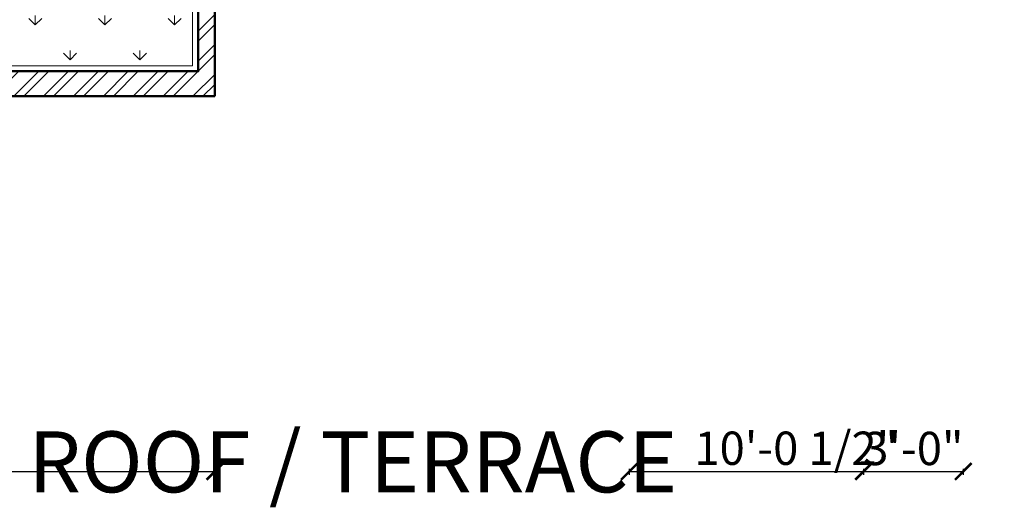
# Model space of a CAD drawing. Units: inches. Extents: x 261 to 2725, y 291 to 1454.
# Tile 27 of 35: x 2144 to 2500, y 291 to 467. Entities that reach past the tile are written whole.
import ezdxf

# ---------------------------------------------------------------- set-up
doc = ezdxf.new("R2010")
doc.units = ezdxf.units.IN
for name, color, linetype, lineweight in [('A-ANNO-DIMS', 136, 'Continuous', 18), ('A-ANNO-TEXT', 7, 'Continuous', 25), ('A-PLNT', 3, 'Continuous', 18), ('A-PLNT-PATT', 3, 'Continuous', 13), ('A-WALL', 222, 'Continuous', 50), ('A-WALL-PATT', 243, 'Continuous', 13)]:
    doc.layers.add(name, color=color, linetype=linetype, lineweight=lineweight)
doc.styles.get("Standard").update_dxf_attribs({"font": 'arial.ttf'})
doc.dimstyles.new('ISO-25', dxfattribs={"dimtxt": 12, "dimasz": 6, "dimexe": 1.25, "dimexo": 0.625, "dimtad": 1, "dimdec": 0, "dimlunit": 3, "dimtxsty": 'Standard', "dimblk": 'ARCHTICK', "dimcen": 2.5, "dimadec": 0, "dimazin": 0, "dimtfac": 1, "dimtdec": 0, "dimtmove": 0, "dimatfit": 3, "dimfxl": 1, "dimfxlon": 1, "dimarcsym": 0})

# ---------------------------------------------------------------- blocks, each defined once
blk = doc.blocks.new('_ArchTick')
at = {"color": 0, "linetype": 'ByBlock', "const_width": 0.15}
blk.add_lwpolyline([(-0.5, -0.5), (0.5, 0.5)], dxfattribs=at)
blk = doc.blocks.new('*D89')
at = {"layer": 'A-ANNO-DIMS', "color": 0, "lineweight": -2, "ltscale": 0.07, "transparency": 16777216}
for p, q in [((2600.96, 508.47), (2603.21, 508.47)), ((2601.96, 412.47), (2601.96, 508.47)), ((2600.96, 412.47), (2603.21, 412.47))]:
    blk.add_line(p, q, dxfattribs=at)
at = {"layer": 'Defpoints', "color": 0, "ltscale": 0.07, "transparency": 16777216}
for p in [(955.45, 508.47), (2601.96, 508.47), (994.45, 412.47)]:
    blk.add_point(p, dxfattribs=at)
at = {"layer": 'A-ANNO-DIMS', "color": 0, "lineweight": -2, "ltscale": 0.07, "transparency": 16777216, "xscale": 6, "yscale": 6, "zscale": 6}
for p, rotation in [((2601.96, 508.47), 90), ((2601.96, 412.47), 270)]:
    blk.add_blockref('_ArchTick', p, dxfattribs=dict(at, rotation=rotation))
at = {"layer": 'A-ANNO-DIMS', "color": 0, "ltscale": 0.07, "transparency": 16777216, "insert": (2595.21, 460.47), "char_height": 12, "attachment_point": 5, "rotation": 90}
blk.add_mtext('8\'-0"', dxfattribs=at)
blk = doc.blocks.new('*D111')
at = {"layer": 'A-ANNO-DIMS', "color": 0, "lineweight": -2, "ltscale": 0.07, "transparency": 16777216}
for p, q in [((2600.96, 550.47), (2603.21, 550.47)), ((2601.96, 448.47), (2601.96, 550.47)), ((2600.96, 448.47), (2603.21, 448.47))]:
    blk.add_line(p, q, dxfattribs=at)
at = {"layer": 'Defpoints', "color": 0, "ltscale": 0.07, "transparency": 16777216}
for p in [(1720.08, 550.47), (2601.96, 550.47), (1720.08, 448.47)]:
    blk.add_point(p, dxfattribs=at)
at = {"layer": 'A-ANNO-DIMS', "color": 0, "lineweight": -2, "ltscale": 0.07, "transparency": 16777216, "xscale": 6, "yscale": 6, "zscale": 6}
for p, rotation in [((2601.96, 550.47), 90), ((2601.96, 448.47), 270)]:
    blk.add_blockref('_ArchTick', p, dxfattribs=dict(at, rotation=rotation))
at = {"layer": 'A-ANNO-DIMS', "color": 0, "ltscale": 0.07, "transparency": 16777216, "insert": (2595.21, 499.47), "char_height": 12, "attachment_point": 5, "rotation": 90}
blk.add_mtext('8\'-6"', dxfattribs=at)
blk = doc.blocks.new('*D124')
at = {"layer": 'A-ANNO-DIMS', "color": 0, "lineweight": -2, "ltscale": 0.07, "transparency": 16777216}
for p, q in [((2007.71, 305.22), (2007.71, 302.97)), ((2007.71, 304.22), (2214.67, 304.22)), ((2214.67, 305.22), (2214.67, 302.97))]:
    blk.add_line(p, q, dxfattribs=at)
at = {"layer": 'Defpoints', "color": 0, "ltscale": 0.07, "transparency": 16777216}
for p in [(2007.71, 439.47), (2214.67, 439.47), (2214.67, 304.22)]:
    blk.add_point(p, dxfattribs=at)
at = {"layer": 'A-ANNO-DIMS', "color": 0, "lineweight": -2, "ltscale": 0.07, "transparency": 16777216, "xscale": 6, "yscale": 6, "zscale": 6, "rotation": 180}
blk.add_blockref('_ArchTick', (2007.71, 304.22), dxfattribs=at)
at = {"layer": 'A-ANNO-DIMS', "color": 0, "lineweight": -2, "ltscale": 0.07, "transparency": 16777216, "xscale": 6, "yscale": 6, "zscale": 6}
blk.add_blockref('_ArchTick', (2214.67, 304.22), dxfattribs=at)
at = {"layer": 'A-ANNO-DIMS', "color": 0, "ltscale": 0.07, "transparency": 16777216, "insert": (2111.19, 310.97), "char_height": 12, "attachment_point": 5}
blk.add_mtext('17\'-3"', dxfattribs=at)
blk = doc.blocks.new('*D125')
at = {"layer": 'A-ANNO-DIMS', "color": 0, "lineweight": -2, "ltscale": 0.07, "transparency": 16777216}
for p, q in [((2600.96, 496.47), (2603.21, 496.47)), ((2601.96, 439.47), (2601.96, 496.47)), ((2600.96, 439.47), (2603.21, 439.47))]:
    blk.add_line(p, q, dxfattribs=at)
at = {"layer": 'Defpoints', "color": 0, "ltscale": 0.07, "transparency": 16777216}
for p in [(2214.67, 496.47), (2601.96, 496.47), (2214.67, 439.47)]:
    blk.add_point(p, dxfattribs=at)
at = {"layer": 'A-ANNO-DIMS', "color": 0, "lineweight": -2, "ltscale": 0.07, "transparency": 16777216, "xscale": 6, "yscale": 6, "zscale": 6}
for p, rotation in [((2601.96, 496.47), 90), ((2601.96, 439.47), 270)]:
    blk.add_blockref('_ArchTick', p, dxfattribs=dict(at, rotation=rotation))
at = {"layer": 'A-ANNO-DIMS', "color": 0, "ltscale": 0.07, "transparency": 16777216, "insert": (2595.21, 467.97), "char_height": 12, "attachment_point": 5, "rotation": 90}
blk.add_mtext('4\'-9"', dxfattribs=at)
blk = doc.blocks.new('*D131')
at = {"layer": 'A-ANNO-DIMS', "color": 0, "lineweight": -2, "ltscale": 0.07, "transparency": 16777216}
for p, q in [((2448.71, 305.22), (2448.71, 302.97)), ((2448.71, 304.22), (2484.71, 304.22)), ((2484.71, 305.22), (2484.71, 302.97))]:
    blk.add_line(p, q, dxfattribs=at)
at = {"layer": 'Defpoints', "color": 0, "ltscale": 0.07, "transparency": 16777216}
for p in [(2448.71, 671.47), (2484.71, 673.47), (2484.71, 304.22)]:
    blk.add_point(p, dxfattribs=at)
at = {"layer": 'A-ANNO-DIMS', "color": 0, "lineweight": -2, "ltscale": 0.07, "transparency": 16777216, "xscale": 6, "yscale": 6, "zscale": 6, "rotation": 180}
blk.add_blockref('_ArchTick', (2448.71, 304.22), dxfattribs=at)
at = {"layer": 'A-ANNO-DIMS', "color": 0, "lineweight": -2, "ltscale": 0.07, "transparency": 16777216, "xscale": 6, "yscale": 6, "zscale": 6}
blk.add_blockref('_ArchTick', (2484.71, 304.22), dxfattribs=at)
at = {"layer": 'A-ANNO-DIMS', "color": 0, "ltscale": 0.07, "transparency": 16777216, "insert": (2466.71, 310.97), "char_height": 12, "attachment_point": 5}
blk.add_mtext('3\'-0"', dxfattribs=at)
blk = doc.blocks.new('*D132')
at = {"layer": 'A-ANNO-DIMS', "color": 0, "lineweight": -2, "ltscale": 0.07, "transparency": 16777216}
for p, q in [((2364.21, 305.22), (2364.21, 302.97)), ((2364.21, 304.22), (2484.71, 304.22)), ((2484.71, 305.22), (2484.71, 302.97))]:
    blk.add_line(p, q, dxfattribs=at)
at = {"layer": 'Defpoints', "color": 0, "ltscale": 0.07, "transparency": 16777216}
for p in [(2364.21, 799.47), (2484.71, 799.47), (2484.71, 304.22)]:
    blk.add_point(p, dxfattribs=at)
at = {"layer": 'A-ANNO-DIMS', "color": 0, "lineweight": -2, "ltscale": 0.07, "transparency": 16777216, "xscale": 6, "yscale": 6, "zscale": 6, "rotation": 180}
blk.add_blockref('_ArchTick', (2364.21, 304.22), dxfattribs=at)
at = {"layer": 'A-ANNO-DIMS', "color": 0, "lineweight": -2, "ltscale": 0.07, "transparency": 16777216, "xscale": 6, "yscale": 6, "zscale": 6}
blk.add_blockref('_ArchTick', (2484.71, 304.22), dxfattribs=at)
at = {"layer": 'A-ANNO-DIMS', "color": 0, "ltscale": 0.07, "transparency": 16777216, "insert": (2424.46, 311.05), "char_height": 12, "attachment_point": 5}
blk.add_mtext('10\'-0 1/2"', dxfattribs=at)

msp = doc.modelspace()

# ---------------------------------------------------------------- hatches: boundary and pattern name
at = {"layer": 'A-PLNT-PATT'}
h = msp.add_hatch(dxfattribs=at)
h.set_pattern_fill('GRASS', color=256, scale=0.7)
h.paths.add_polyline_path([(2052.71, 797.47), (2018.71, 797.47), (2018.71, 450.47), (2206.67, 450.47), (2206.67, 507.47), (2482.71, 507.47), (2482.71, 671.47), (2448.71, 671.47), (2448.71, 541.47), (2172.67, 541.47), (2172.67, 484.47), (2052.71, 484.47)])
at = {"layer": 'A-WALL-PATT'}
h = msp.add_hatch(dxfattribs=at)
h.set_pattern_fill('ANSI32', color=256, scale=0.8)
h.paths.add_polyline_path([(478.45, 685.47), (580.45, 685.47), (580.45, 691.47), (577.45, 691.47), (577.45, 694.47), (571.45, 694.47), (571.45, 691.47), (478.45, 691.47), (478.45, 721.47), (469.45, 721.47), (469.45, 508.47), (538.45, 508.47), (538.45, 517.47), (478.45, 517.47)])
h.paths.add_polyline_path([(694.45, 517.47), (676.45, 517.47), (676.45, 646.47), (670.45, 646.47), (670.45, 517.47), (610.45, 517.47), (610.45, 508.47), (694.45, 508.47)])
h.paths.add_polyline_path([(676.45, 784.47), (478.45, 784.47), (478.45, 844.47), (469.45, 844.47), (469.45, 745.47), (478.45, 745.47), (478.45, 775.47), (571.45, 775.47), (571.45, 724.47), (577.45, 724.47), (577.45, 775.47), (670.45, 775.47), (670.45, 691.47), (610.45, 691.47), (610.45, 685.47), (670.45, 685.47), (670.45, 682.47), (676.45, 682.47)])
h.paths.add_polyline_path([(955.45, 880.47), (946.45, 880.47), (946.45, 808.47), (778.45, 808.47), (778.45, 799.47), (946.45, 799.47), (946.45, 517.47), (898.45, 517.47), (898.45, 508.47), (955.45, 508.47)])
h.paths.add_polyline_path([(778.45, 598.47), (772.45, 598.47), (772.45, 517.47), (754.45, 517.47), (754.45, 508.47), (826.45, 508.47), (826.45, 517.47), (778.45, 517.47)])
h.paths.add_polyline_path([(955.45, 1090.47), (946.45, 1090.47), (946.45, 1030.47), (817.45, 1030.47), (817.45, 1024.47), (946.45, 1024.47), (946.45, 952.47), (955.45, 952.47)])
h.paths.add_polyline_path([(955.45, 1231.47), (730.45, 1231.47), (730.45, 1222.47), (772.45, 1222.47), (772.45, 1096.47), (766.45, 1096.47), (766.45, 1090.47), (772.45, 1090.47), (772.45, 1006.47), (712.45, 1006.47), (712.45, 1000.47), (778.45, 1000.47), (778.45, 1024.47), (781.45, 1024.47), (781.45, 1030.47), (778.45, 1030.47), (778.45, 1222.47), (946.45, 1222.47), (946.45, 1162.47), (955.45, 1162.47)])
h.paths.add_polyline_path([(694.45, 1231.47), (619.45, 1231.47), (619.45, 1222.47), (646.45, 1222.47), (646.45, 1039.47), (652.45, 1039.47), (652.45, 1090.47), (736.45, 1090.47), (736.45, 1096.47), (652.45, 1096.47), (652.45, 1222.47), (694.45, 1222.47)])
h.paths.add_polyline_path([(571.45, 1231.47), (469.45, 1231.47), (469.45, 1099.47), (478.45, 1099.47), (478.45, 1144.47), (544.45, 1144.47), (544.45, 1153.47), (538.45, 1153.47), (538.45, 1150.47), (478.45, 1150.47), (478.45, 1222.47), (538.45, 1222.47), (538.45, 1183.47), (544.45, 1183.47), (544.45, 1222.47), (571.45, 1222.47)])
h.paths.add_polyline_path([(538.45, 1006.47), (478.45, 1006.47), (478.45, 1051.47), (469.45, 1051.47), (469.45, 940.47), (478.45, 940.47), (478.45, 1000.47), (538.45, 1000.47)])
h.paths.add_polyline_path([(652.45, 1006.47), (652.45, 1009.47), (646.45, 1009.47), (646.45, 1006.47), (586.45, 1006.47), (586.45, 1000.47), (652.45, 1000.47)])
h.paths.add_polyline_path([(1288.08, 973.47), (1243.08, 973.47), (1243.08, 920.97), (1252.08, 920.97), (1252.08, 964.47), (1288.08, 964.47)], flags=17)
h.paths.add_polyline_path([(1402.08, 805.47), (1252.08, 805.47), (1252.08, 848.97), (1243.08, 848.97), (1243.08, 757.47), (1252.08, 757.47), (1252.08, 799.47), (1294.08, 799.47), (1372.08, 799.47), (1372.08, 779.47), (1372.08, 715.47), (1378.08, 715.47), (1378.08, 799.47), (1402.08, 799.47)])
h.paths.add_polyline_path([(1252.08, 721.47), (1243.08, 721.47), (1243.08, 439.47), (1729.08, 439.47), (1729.08, 709.47), (1720.08, 709.47), (1720.08, 679.47), (1582.08, 679.47), (1582.08, 670.47), (1588.08, 670.47), (1588.08, 673.47), (1720.08, 673.47), (1720.08, 559.47), (1690.08, 559.47), (1690.08, 550.47), (1720.08, 550.47), (1720.08, 448.47), (1252.08, 448.47), (1252.08, 496.47), (1312.08, 496.47), (1312.08, 505.47), (1252.08, 505.47), (1252.08, 673.47), (1405.08, 673.47), (1405.08, 679.47), (1378.08, 679.47), (1378.08, 685.47), (1372.08, 685.47), (1372.08, 679.47), (1252.08, 679.47)])
h.paths.add_polyline_path([(1450.08, 550.47), (1480.08, 550.47), (1480.08, 559.47), (1450.08, 559.47), (1450.08, 679.47), (1441.08, 679.47), (1441.08, 673.47), (1444.08, 673.47), (1444.08, 505.47), (1384.08, 505.47), (1384.08, 496.47), (1450.08, 496.47)], flags=17)
h.paths.add_polyline_path([(1618.08, 559.47), (1588.08, 559.47), (1588.08, 634.47), (1582.08, 634.47), (1582.08, 559.47), (1552.08, 559.47), (1552.08, 550.47), (1618.08, 550.47)], flags=17)
h.paths.add_polyline_path([(1564.08, 964.47), (1630.08, 964.47), (1630.08, 973.47), (1477.08, 973.47), (1477.08, 964.47), (1558.08, 964.47), (1558.08, 926.22), (1558.08, 887.97), (1486.08, 887.97), (1486.08, 881.97), (1558.08, 881.97), (1558.08, 805.47), (1450.08, 805.47), (1450.08, 845.97), (1444.08, 845.97), (1444.08, 805.47), (1438.08, 805.47), (1438.08, 799.47), (1564.08, 799.47)], flags=17)
h.paths.add_polyline_path([(1453.08, 973.47), (1408.08, 973.47), (1408.08, 964.47), (1444.08, 964.47), (1444.08, 881.97), (1450.08, 881.97), (1456.08, 881.97), (1456.08, 887.97), (1450.08, 887.97), (1450.08, 964.47), (1453.08, 964.47)], flags=17)
h.paths.add_polyline_path([(1729.08, 1231.47), (1243.08, 1231.47), (1243.08, 1167.47), (1252.08, 1167.47), (1252.08, 1222.47), (1441.08, 1222.47), (1441.08, 1045.47), (1648.08, 1045.47), (1648.08, 1051.47), (1450.08, 1051.47), (1450.08, 1074.47), (1450.08, 1222.47), (1472.08, 1222.47), (1720.08, 1222.47), (1720.08, 1051.47), (1708.08, 1051.47), (1708.08, 1045.47), (1720.08, 1045.47), (1720.08, 973.47), (1702.08, 973.47), (1702.08, 964.47), (1720.08, 964.47), (1720.08, 769.47), (1729.08, 769.47)])
h.paths.add_polyline_path([(2493.71, 1054.85), (2007.71, 1054.85), (2007.71, 439.47), (2214.67, 439.47), (2214.67, 496.47), (2493.71, 496.47)])
h.paths.add_polyline_path([(2016.71, 1045.85), (2304.71, 1045.85), (2304.71, 841.47), (2310.71, 841.47), (2310.71, 1045.85), (2484.71, 1045.85), (2484.71, 805.47), (2310.71, 805.47), (2310.71, 811.47), (2304.71, 811.47), (2304.71, 799.47), (2484.71, 799.47), (2484.71, 679.47), (2304.71, 679.47), (2304.71, 673.47), (2484.71, 673.47), (2484.71, 505.47), (2208.67, 505.47), (2208.67, 448.47), (2016.71, 448.47), (2016.71, 799.47), (2304.71, 799.47), (2304.71, 805.47), (2016.71, 805.47)], flags=16)

# ---------------------------------------------------------------- linework, layer by layer
at = {"layer": 'A-PLNT'}
msp.add_lwpolyline([(2018.71, 797.47), (2018.71, 450.47), (2206.67, 450.47), (2206.67, 507.47), (2482.71, 507.47), (2482.71, 671.47)], dxfattribs=at)
at = {"layer": 'A-WALL'}
for p in [(2214.67, 496.47), (2007.71, 439.47)]:
    msp.add_line(p, (2214.67, 439.47), dxfattribs=at)
msp.add_lwpolyline([(2016.71, 799.47), (2016.71, 448.47), (2208.67, 448.47), (2208.67, 505.47), (2484.71, 505.47), (2484.71, 673.47)], dxfattribs=at)

# ---------------------------------------------------------------- texts
at = {"layer": 'A-ANNO-TEXT', "insert": (2134.07, 318.69), "char_height": 22, "attachment_point": 1}
msp.add_mtext_dynamic_manual_height_columns('\\pxqc;{\\fTimes New Roman|b0|i0|c0|p18;ROOF / TERRACE}', width=260.751, gutter_width=12.5, heights=[0], dxfattribs=at)

# ---------------------------------------------------------------- dimensions: what is measured, and where the dimension line sits
at = {"layer": 'A-ANNO-DIMS', "ltscale": 0.07}
for base, p1, p2, picture, middle in [((2484.71, 304.22), (2364.21, 799.47), (2484.71, 799.47), '*D132', (2424.46, 311.05)), ((2484.71, 304.22), (2448.71, 671.47), (2484.71, 673.47), '*D131', (2466.71, 310.97)), ((2214.67, 304.22), (2007.71, 439.47), (2214.67, 439.47), '*D124', (2111.19, 310.97))]:
    dim = msp.add_linear_dim(base=base, p1=p1, p2=p2, dimstyle='ISO-25', override={"dimdec": 1, "dimlfac": 1, "dimrnd": 0, "dimzin": 1, "dimdsep": 46, "dimlunit": 4, "dimfrac": 2}, dxfattribs=at)
    dim.commit()
    dim.dimension.update_dxf_attribs({"geometry": picture, "text_midpoint": middle})
for base, p1, p2, picture, middle in [((2601.96, 550.47), (1720.08, 448.47), (1720.08, 550.47), '*D111', (2595.21, 499.47)), ((2601.96, 508.47), (994.45, 412.47), (955.45, 508.47), '*D89', (2595.21, 460.47)), ((2601.96, 496.47), (2214.67, 439.47), (2214.67, 496.47), '*D125', (2595.21, 467.97))]:
    dim = msp.add_linear_dim(base=base, p1=p1, p2=p2, angle=90, dimstyle='ISO-25', override={"dimdec": 1, "dimlfac": 1, "dimrnd": 0, "dimzin": 1, "dimdsep": 46, "dimlunit": 4, "dimfrac": 2}, dxfattribs=at)
    dim.commit()
    dim.dimension.update_dxf_attribs({"geometry": picture, "text_midpoint": middle})

doc.saveas('drawing.dxf')
